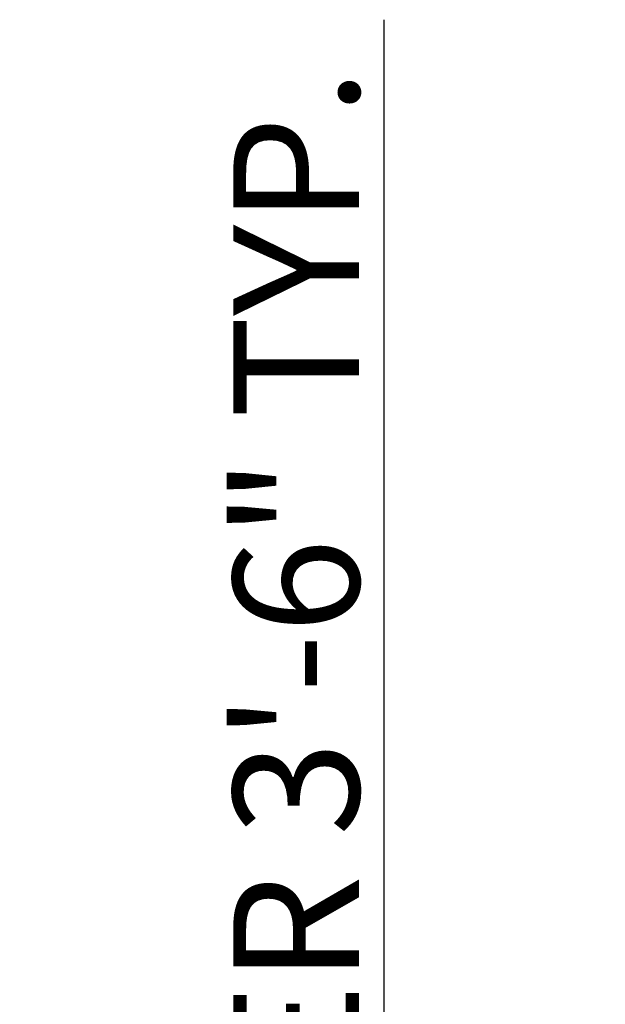
# Model space of a CAD drawing. Units: millimetres. Extents: x 542930 to 543750, y 628093 to 628738.
# Tile 13 of 14: x 543374 to 543429, y 628644 to 628738. Entities that reach past the tile are written whole.
import ezdxf

# ---------------------------------------------------------------- set-up
doc = ezdxf.new("R2010")
doc.units = ezdxf.units.MM
doc.layers.add('A-ANNO-DIMS', color=2, linetype='Continuous', lineweight=18)
doc.styles.get("Standard").update_dxf_attribs({"font": 'arial.ttf'})
doc.dimstyles.new('ISO-25', dxfattribs={"dimtxt": 12, "dimasz": 2.5, "dimexe": 1.25, "dimexo": 0.625, "dimtad": 1, "dimdec": 0, "dimlunit": 3, "dimtxsty": 'Standard', "dimcen": 2.5, "dimadec": 0, "dimazin": 0, "dimtfac": 1, "dimtdec": 0, "dimtmove": 0, "dimatfit": 3, "dimfxl": 1, "dimarcsym": 0})

# ---------------------------------------------------------------- blocks, each defined once
blk = doc.blocks.new('*D53')
at = {"layer": 'A-ANNO-DIMS', "color": 0, "lineweight": -2, "transparency": 16777216}
for p, q in [((543408.367, 628580.826), (543408.367, 628737.76)), ((543414.042, 628580.826), (543407.117, 628580.826)), ((543408.367, 628541.326), (543408.367, 628578.326)), ((543414.042, 628538.826), (543407.117, 628538.826))]:
    blk.add_line(p, q, dxfattribs=at)
at = {"layer": 'A-ANNO-DIMS', "color": 0, "transparency": 16777216}
for points in [[(543407.95, 628578.326), (543408.784, 628578.326), (543408.367, 628580.826)], [(543407.95, 628541.326), (543408.784, 628541.326), (543408.367, 628538.826)]]:
    blk.add_solid(points, dxfattribs=at)
at = {"layer": 'Defpoints', "color": 0, "transparency": 16777216}
for p in [(543408.367, 628580.826), (543414.667, 628580.826), (543414.667, 628538.826)]:
    blk.add_point(p, dxfattribs=at)
at = {"layer": 'A-ANNO-DIMS', "color": 0, "transparency": 16777216, "insert": (543401.529, 628660.543), "char_height": 12, "attachment_point": 5, "rotation": 90}
blk.add_mtext('SHOWER 3\'-6" TYP.', dxfattribs=at)

msp = doc.modelspace()

# ---------------------------------------------------------------- dimensions: what is measured, and where the dimension line sits
at = {"layer": 'A-ANNO-DIMS'}
dim = msp.add_linear_dim(base=(543408.367, 628580.826), p1=(543414.667, 628538.826), p2=(543414.667, 628580.826), angle=90, text='SHOWER <> TYP.', dimstyle='ISO-25', override={"dimdec": 1, "dimlfac": 1, "dimrnd": 0, "dimzin": 1, "dimdsep": 46, "dimlunit": 4, "dimfrac": 2}, dxfattribs=at)
dim.commit()
dim.dimension.update_dxf_attribs({"geometry": '*D53', "text_midpoint": (543401.529, 628660.543)})

doc.saveas('drawing.dxf')
